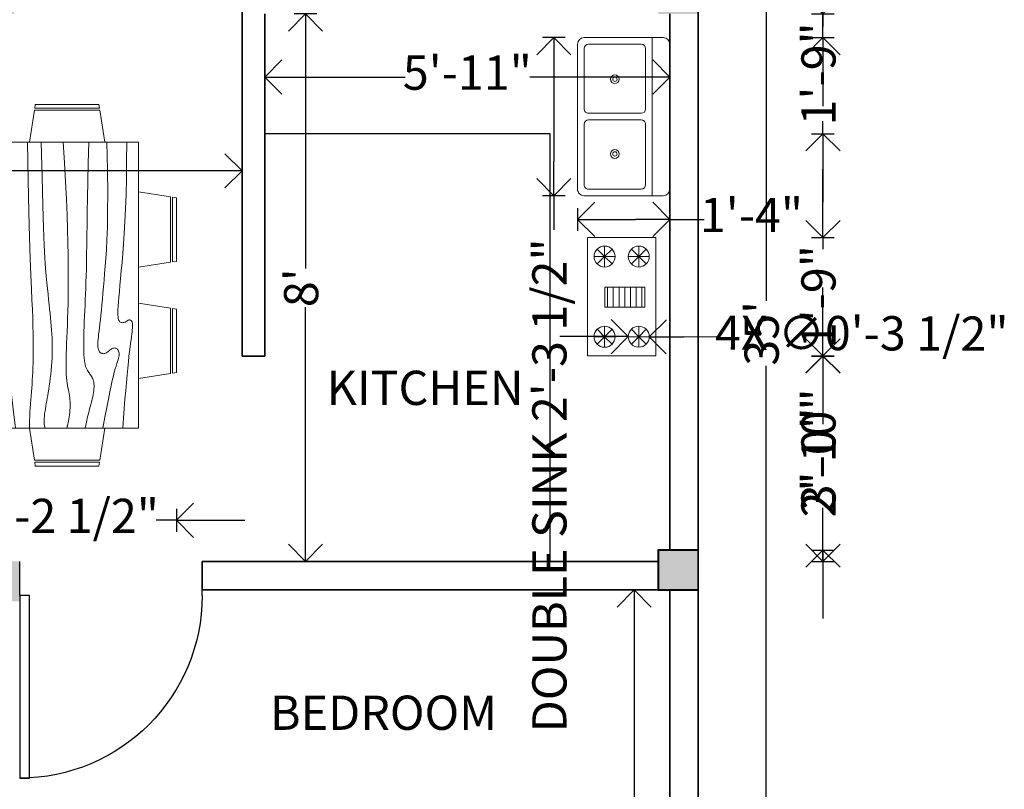
# Model space of a CAD drawing. Units: inches. Extents: x 261 to 714, y 97 to 573.
# Tile 4 of 5: x 541 to 714, y 253 to 388. Entities that reach past the tile are written whole.
import ezdxf

# ---------------------------------------------------------------- set-up
doc = ezdxf.new("R2010")
doc.units = ezdxf.units.IN
for name, color, linetype, lineweight in [('A-ANNO-DIMS', 2, 'Continuous', 18), ('A-AREA-IDEN', 7, 'Continuous', 25), ('A-COLS', 182, 'Continuous', 40), ('A-COLS-PATT', 172, 'Continuous', 13), ('A-DOOR', 182, 'Continuous', 25), ('A-EQPM', 8, 'Continuous', 18), ('A-FLOR-CASE', 182, 'Continuous', 25), ('A-FLOR-FIXT', 8, 'Continuous', 18), ('A-FURN', 8, 'Continuous', 18), ('A-WALL', 182, 'Continuous', 35)]:
    doc.layers.add(name, color=color, linetype=linetype, lineweight=lineweight)
doc.styles.get("Standard").update_dxf_attribs({"font": 'arial.ttf'})
doc.dimstyles.new('ISO-25', dxfattribs={"dimtxt": 6, "dimasz": 6, "dimexe": 2, "dimexo": 2, "dimtad": 0, "dimdec": 1, "dimlunit": 3, "dimtxsty": 'Standard', "dimblk": 'OPEN90', "dimcen": 2.5, "dimclrd": 1, "dimclre": 1, "dimclrt": 1, "dimadec": 0, "dimazin": 0, "dimtfac": 1, "dimtdec": 1, "dimtmove": 0, "dimatfit": 3, "dimfxl": 2, "dimfxlon": 1, "dimarcsym": 0})

# ---------------------------------------------------------------- blocks, each defined once
blk = doc.blocks.new('*U5')
for p, q in [((0, 0), (0, -6)), ((32, 0), (32, -6))]:
    blk.add_line(p, q)
blk.add_lwpolyline([(0, 0), (0, 32), (1.75, 32), (1.75, 0)], close=True)
blk.add_arc((0, 0), 32, 0, 90)
blk = doc.blocks.new('_Open90')
at = {"color": 0, "linetype": 'ByBlock', "lineweight": -2}
for p, q in [((-0.5, 0.5), (0, 0)), ((0, 0), (-1, 0)), ((0, 0), (-0.5, -0.5))]:
    blk.add_line(p, q, dxfattribs=at)
blk = doc.blocks.new('*D15')
at = {"layer": 'A-ANNO-DIMS', "color": 0, "lineweight": -2, "transparency": 16777216}
for p, q in [((352.9, 361.16), (352.9, 359.16)), ((358.9, 361.16), (453.42, 361.16)), ((573.9, 361.16), (479.38, 361.16)), ((579.9, 361.16), (579.9, 359.16))]:
    blk.add_line(p, q, dxfattribs=at)
at = {"layer": 'Defpoints', "color": 0, "transparency": 16777216}
for p in [(352.9, 361.54), (579.9, 361.54), (579.9, 361.16)]:
    blk.add_point(p, dxfattribs=at)
at = {"layer": 'A-ANNO-DIMS', "color": 0, "lineweight": -2, "transparency": 16777216, "xscale": 6, "yscale": 6, "zscale": 6, "rotation": 180}
blk.add_blockref('_Open90', (352.9, 361.16), dxfattribs=at)
at = {"layer": 'A-ANNO-DIMS', "color": 0, "lineweight": -2, "transparency": 16777216, "xscale": 6, "yscale": 6, "zscale": 6}
blk.add_blockref('_Open90', (579.9, 361.16), dxfattribs=at)
at = {"layer": 'A-ANNO-DIMS', "color": 0, "transparency": 16777216, "insert": (466.4, 361.16), "char_height": 6, "attachment_point": 5}
blk.add_mtext('18\'-10"', dxfattribs=at)
blk = doc.blocks.new('*D17')
at = {"layer": 'A-ANNO-DIMS', "color": 0, "lineweight": -2, "transparency": 16777216}
for p, q in [((593.03, 388.66), (589.03, 388.66)), ((591.03, 382.66), (591.03, 344.05)), ((591.03, 298.66), (591.03, 337.27)), ((593.03, 292.66), (589.03, 292.66))]:
    blk.add_line(p, q, dxfattribs=at)
at = {"layer": 'Defpoints', "color": 0, "transparency": 16777216}
for p in [(649.85, 388.66), (591.03, 292.66), (649.85, 292.66)]:
    blk.add_point(p, dxfattribs=at)
at = {"layer": 'A-ANNO-DIMS', "color": 0, "lineweight": -2, "transparency": 16777216, "xscale": 6, "yscale": 6, "zscale": 6}
for p, rotation in [((591.03, 388.66), 90), ((591.03, 292.66), 270)]:
    blk.add_blockref('_Open90', p, dxfattribs=dict(at, rotation=rotation))
at = {"layer": 'A-ANNO-DIMS', "color": 0, "transparency": 16777216, "insert": (591.03, 340.66), "char_height": 6, "attachment_point": 5, "rotation": 90}
blk.add_mtext("8'", dxfattribs=at)
blk = doc.blocks.new('*D18')
at = {"layer": 'A-ANNO-DIMS', "color": 0, "lineweight": -2, "transparency": 16777216}
for p, q in [((583.9, 375.6), (583.9, 379.6)), ((654.9, 375.6), (654.9, 379.6)), ((589.9, 377.6), (608.47, 377.6)), ((648.9, 377.6), (630.33, 377.6))]:
    blk.add_line(p, q, dxfattribs=at)
at = {"layer": 'Defpoints', "color": 0, "transparency": 16777216}
for p in [(654.9, 377.6), (583.9, 358.66), (654.9, 358.66)]:
    blk.add_point(p, dxfattribs=at)
at = {"layer": 'A-ANNO-DIMS', "color": 0, "lineweight": -2, "transparency": 16777216, "xscale": 6, "yscale": 6, "zscale": 6, "rotation": 180}
blk.add_blockref('_Open90', (583.9, 377.6), dxfattribs=at)
at = {"layer": 'A-ANNO-DIMS', "color": 0, "lineweight": -2, "transparency": 16777216, "xscale": 6, "yscale": 6, "zscale": 6}
blk.add_blockref('_Open90', (654.9, 377.6), dxfattribs=at)
at = {"layer": 'A-ANNO-DIMS', "color": 0, "transparency": 16777216, "insert": (619.4, 377.6), "char_height": 6, "attachment_point": 5}
blk.add_mtext('5\'-11"', dxfattribs=at)
blk = doc.blocks.new('*D21')
at = {"layer": 'A-ANNO-DIMS', "color": 0, "lineweight": -2, "transparency": 16777216}
for p, q in [((646.66, 287.66), (650.66, 287.66)), ((648.66, 281.66), (648.66, 233.09)), ((648.66, 173.66), (648.66, 222.22)), ((646.66, 167.66), (650.66, 167.66))]:
    blk.add_line(p, q, dxfattribs=at)
at = {"layer": 'Defpoints', "color": 0, "transparency": 16777216}
for p in [(643.84, 287.66), (643.84, 167.66), (648.66, 167.66)]:
    blk.add_point(p, dxfattribs=at)
at = {"layer": 'A-ANNO-DIMS', "color": 0, "lineweight": -2, "transparency": 16777216, "xscale": 6, "yscale": 6, "zscale": 6}
for p, rotation in [((648.66, 287.66), 90), ((648.66, 167.66), 270)]:
    blk.add_blockref('_Open90', p, dxfattribs=dict(at, rotation=rotation))
at = {"layer": 'A-ANNO-DIMS', "color": 0, "transparency": 16777216, "insert": (648.66, 227.66), "char_height": 6, "attachment_point": 5, "rotation": 90}
blk.add_mtext("10'", dxfattribs=at)
blk = doc.blocks.new('Sink-double - 36 in top')
for p, q in [((-18, -4), (18, -4)), ((-0.75, -18.5), (-0.75, -6.5)), ((0.75, -6.5), (0.75, -18.5))]:
    blk.add_line(p, q)
for points in [[(-16.5, 0), (16.5, 0)], [(-18, -19.5), (-18, -1.5)], [(18, -1.5), (18, -19.5)], [(-16.5, -18.5), (-16.5, -6.5)], [(-15.5, -5.5), (-1.75, -5.5)], [(1.75, -5.5), (15.5, -5.5)], [(16.5, -6.5), (16.5, -18.5)], [(-1.75, -19.5), (-15.5, -19.5)], [(15.5, -19.5), (1.75, -19.5)], [(16.5, -21), (-16.5, -21)]]:
    blk.add_lwpolyline(points)
for centre, radius in [((-8.5, -12.5), 1), ((-8.5, -12.5), 0.5), ((8.5, -12.5), 1), ((8.5, -12.5), 0.5)]:
    blk.add_circle(centre, radius)
for centre, radius, start, end in [((-16.5, -1.5), 1.5, 90, 180), ((16.5, -1.5), 1.5, 0, 90), ((-15.5, -6.5), 1, 90, 180), ((-1.75, -6.5), 1, 0, 90), ((1.75, -6.5), 1, 90, 180), ((15.5, -6.5), 1, 0, 90), ((-16.5, -19.5), 1.5, 180, 270), ((-15.5, -18.5), 1, 180, 270), ((-1.75, -18.5), 1, 270, 0), ((1.75, -18.5), 1, 180, 270), ((15.5, -18.5), 1, 270, 0), ((16.5, -19.5), 1.5, 270, 0)]:
    blk.add_arc(centre, radius, start, end)
blk = doc.blocks.new('Dining Set - 36 x 72 in.')
for p, q in [((-22, 27.5), (-22.1562, 26.50042)), ((-22, 27.5), (-6, 27.5)), ((-5.8437, 26.49966), (-6, 27.5)), ((6, 27.5), (5.8438, 26.50042)), ((6, 27.5), (22, 27.5)), ((22.1563, 26.49966), (22, 27.5)), ((-22.2343, 26.00059), (-23.4847, 17.99762)), ((-22.2304, 26), (-5.7608, 26)), ((-5.8416, 26.5), (-22.1534, 26.5)), ((-4.5152, 17.99762), (-5.7655, 25.99926)), ((5.7657, 26.00059), (4.5153, 17.99762)), ((5.7696, 26), (22.2392, 26)), ((22.1584, 26.5), (5.8466, 26.5)), ((23.4848, 17.99762), (22.2345, 25.99926)), ((36, 18), (-36, 18)), ((-36, 18), (-36, -18)), ((36, -18), (36, 18)), ((-45.5, 8), (-44.5004, 8.15617)), ((-45.5, 8), (-45.5, -8)), ((-44.5, -8.15843), (-44.5, 8.15338)), ((-44.0006, 8.23428), (-35.9976, 9.48474)), ((-44, 8.23041), (-44, -8.23915)), ((44.0006, 8.23428), (35.9976, 9.48474)), ((44, 8.23041), (44, -8.23915)), ((44.5, -8.15843), (44.5, 8.15338)), ((45.5, 8), (44.5005, 8.15617)), ((45.5, 8), (45.5, -8)), ((-44.4997, -8.15631), (-45.5, -8)), ((-35.9976, -9.48476), (-43.9993, -8.2345)), ((35.9976, -9.48476), (43.9993, -8.2345)), ((44.4997, -8.15631), (45.5, -8)), ((-36, -18), (36, -18)), ((-22.2343, -26.0006), (-23.4847, -17.99762)), ((-4.5152, -17.99762), (-5.7655, -25.99928)), ((5.7657, -26.0006), (4.5153, -17.99762)), ((23.4848, -17.99762), (22.2345, -25.99928)), ((-22.2304, -26), (-5.7608, -26)), ((-22, -27.5), (-22.1562, -26.50044)), ((-5.8416, -26.5), (-22.1534, -26.5)), ((-5.8437, -26.49967), (-6, -27.5)), ((5.7696, -26), (22.2392, -26)), ((6, -27.5), (5.8438, -26.50044)), ((22.1584, -26.5), (5.8466, -26.5)), ((22.1563, -26.49967), (22, -27.5)), ((-22, -27.5), (-6, -27.5)), ((6, -27.5), (22, -27.5))]:
    blk.add_line(p, q)
for points in [[(-36, 15), (-31.1772, 14.97754), (-26.8079, 14.91406), (-22.8538, 14.81543), (-19.276, 14.6875), (-16.0362, 14.53613), (-13.0957, 14.36718), (-10.4159, 14.18652), (-7.9583, 14), (-5.6904, 13.81315), (-3.6035, 13.63021), (-1.6954, 13.45508), (0.0365, 13.29166), (1.5945, 13.14388), (2.9811, 13.01562), (4.1988, 12.9108), (5.25, 12.83333), (6.1393, 12.78613), (6.8802, 12.76823), (7.4883, 12.77767), (7.9792, 12.8125), (8.3685, 12.87077), (8.6719, 12.95052), (8.9049, 13.0498), (9.0833, 13.16666), (9.2205, 13.29899), (9.3216, 13.44401), (9.3895, 13.59879), (9.4271, 13.76041), (9.4373, 13.92594), (9.4232, 14.09245), (9.3875, 14.257), (9.3333, 14.41666), (9.2638, 14.56917), (9.1836, 14.71484), (9.0975, 14.85465), (9.0104, 14.98958), (8.9272, 15.1206), (8.8529, 15.2487), (8.7922, 15.37483), (8.75, 15.5), (8.7305, 15.62467), (8.7344, 15.74739), (8.7617, 15.86621), (8.8125, 15.97916), (8.8867, 16.08431), (8.9844, 16.17968), (9.1055, 16.26334), (9.25, 16.33333), (9.4189, 16.38802), (9.6172, 16.42708), (9.8506, 16.45052), (10.125, 16.45833), (10.4463, 16.45052), (10.8203, 16.42708), (11.2529, 16.38802), (11.75, 16.33333), (12.3184, 16.26318), (12.9694, 16.17838), (13.7151, 16.07991), (14.5677, 15.96875), (15.5395, 15.84586), (16.6426, 15.71224), (17.8893, 15.56884), (19.2917, 15.41666), (20.859, 15.25667), (22.5879, 15.08984), (24.4721, 14.91715), (26.5052, 14.73958), (28.6809, 14.5581), (30.9929, 14.3737), (33.4347, 14.18733), (36, 14)], [(-36, 10), (-28.9766, 10.14274), (-23.1725, 10.20442), (-18.4241, 10.19775), (-14.5677, 10.13541), (-11.4399, 10.03011), (-8.877, 9.89453), (-6.7154, 9.74137), (-4.7917, 9.58333), (-2.9698, 9.43082), (-1.2246, 9.28515), (0.4415, 9.14534), (2.026, 9.01041), (3.5266, 8.87939), (4.9408, 8.7513), (6.266, 8.62516), (7.5, 8.5), (8.6411, 8.37549), (9.6914, 8.2539), (10.6538, 8.13818), (11.5312, 8.03125), (12.3267, 7.93603), (13.043, 7.85547), (13.6831, 7.79248), (14.25, 7.75), (14.7471, 7.7303), (15.1797, 7.73307), (15.5537, 7.75732), (15.875, 7.80208), (16.1494, 7.86637), (16.3828, 7.94922), (16.5811, 8.04964), (16.75, 8.16666), (16.8944, 8.29915), (17.0143, 8.44531), (17.1089, 8.60319), (17.1771, 8.77083), (17.218, 8.94629), (17.2305, 9.1276), (17.2137, 9.31282), (17.1667, 9.5), (17.0895, 9.6875), (16.987, 9.875), (16.8649, 10.0625), (16.7292, 10.25), (16.5856, 10.4375), (16.4401, 10.625), (16.2985, 10.8125), (16.1667, 11), (16.05, 11.18733), (15.9518, 11.3737), (15.8752, 11.5581), (15.8229, 11.73958), (15.798, 11.91715), (15.8034, 12.08984), (15.842, 12.25667), (15.9167, 12.41666), (16.0295, 12.56836), (16.1784, 12.70833), (16.3605, 12.83268), (16.5729, 12.9375), (16.8127, 13.01888), (17.0768, 13.07291), (17.3625, 13.0957), (17.6667, 13.08333), (17.9894, 13.03312), (18.3418, 12.94726), (18.7382, 12.82918), (19.1927, 12.68229), (19.7195, 12.51001), (20.3327, 12.31575), (21.0465, 12.10294), (21.875, 11.875), (22.8357, 11.63354), (23.959, 11.37304), (25.2786, 11.08618), (26.8282, 10.76562), (28.6414, 10.40405), (30.752, 9.99414), (33.1936, 9.52856), (36, 9)], [(-36, 5.5), (-30.7157, 5.3348), (-26.069, 5.20963), (-21.9946, 5.11767), (-18.4271, 5.05208), (-15.3009, 5.00602), (-12.5508, 4.97265), (-10.1112, 4.94515), (-7.9167, 4.91666), (-5.909, 4.88167), (-4.0586, 4.83984), (-2.3429, 4.79215), (-0.7396, 4.73958), (0.7739, 4.6831), (2.22, 4.6237), (3.6213, 4.56233), (5, 4.5), (6.373, 4.43782), (7.7344, 4.3776), (9.0723, 4.32129), (10.375, 4.27083), (11.6309, 4.22819), (12.8281, 4.19531), (13.9551, 4.17415), (15, 4.16666), (15.954, 4.17448), (16.819, 4.19791), (17.6001, 4.23698), (18.3021, 4.29166), (18.9299, 4.36198), (19.4883, 4.44791), (19.9823, 4.54948), (20.4167, 4.66666), (20.7969, 4.79899), (21.1302, 4.94401), (21.4245, 5.09879), (21.6875, 5.26041), (21.9271, 5.42594), (22.1511, 5.59245), (22.3672, 5.757), (22.5834, 5.91666), (22.8065, 6.06868), (23.0404, 6.21093), (23.2879, 6.34147), (23.5521, 6.45833), (23.8358, 6.55957), (24.142, 6.64323), (24.4735, 6.70735), (24.8334, 6.75), (25.2235, 6.76969), (25.642, 6.76692), (26.0858, 6.74267), (26.5521, 6.69791), (27.0379, 6.63362), (27.5404, 6.55078), (28.0565, 6.45036), (28.5834, 6.33333), (29.1242, 6.19987), (29.7071, 6.04687), (30.3661, 5.87044), (31.1354, 5.66666), (32.0493, 5.43164), (33.142, 5.16146), (34.4475, 4.85221), (36, 4.5)], [(-36, -1), (-30.7915, -0.6591), (-26.0195, -0.38216), (-21.6519, -0.16284), (-17.6563, 0.00521), (-14.0005, 0.12833), (-10.6523, 0.21289), (-7.5796, 0.26522), (-4.75, 0.29166), (-2.134, 0.29793), (0.2878, 0.28711), (2.5317, 0.26163), (4.6146, 0.22396), (6.5529, 0.17651), (8.3633, 0.12174), (10.0623, 0.06209), (11.6667, 0), (13.1899, -0.06201), (14.6341, -0.1211), (15.9982, -0.17432), (17.2813, -0.21875), (18.4823, -0.25147), (19.6003, -0.26953), (20.6343, -0.27002), (21.5834, -0.25), (22.4481, -0.20768), (23.2357, -0.14584), (23.9549, -0.06836), (24.6146, 0.02083), (25.2235, 0.11784), (25.7904, 0.21875), (26.3241, 0.31966), (26.8334, 0.41666), (27.3265, 0.50618), (27.8099, 0.58593), (28.2894, 0.65397), (28.7709, 0.70833), (29.2601, 0.74707), (29.763, 0.76823), (30.2855, 0.76985), (30.8334, 0.75), (31.4088, 0.70784), (31.9994, 0.64713), (32.589, 0.57275), (33.1615, 0.48958), (33.7008, 0.4025), (34.1908, 0.3164), (34.6153, 0.23616), (34.9584, 0.16666), (35.2099, 0.11165), (35.3848, 0.07031), (35.504, 0.04069), (35.5886, 0.02083), (35.6594, 0.00879), (35.7377, 0.0026), (35.8442, 0.00032), (36, 0)], [(-36, -6.5), (-27.1843, -6.31267), (-20.084, -6.1263), (-14.469, -5.9419), (-10.1094, -5.76042), (-6.7752, -5.58285), (-4.2363, -5.41016), (-2.2629, -5.24333), (-0.625, -5.08334), (0.8708, -4.93099), (2.2715, -4.78646), (3.5872, -4.64974), (4.8281, -4.52084), (6.0046, -4.39974), (7.127, -4.28646), (8.2053, -4.18099), (9.25, -4.08334), (10.2705, -3.99382), (11.2734, -3.91407), (12.2647, -3.84603), (13.25, -3.79167), (14.2354, -3.75293), (15.2266, -3.73177), (16.2295, -3.73015), (17.25, -3.75), (18.2912, -3.79248), (19.3451, -3.85547), (20.4009, -3.93604), (21.4479, -4.03125), (22.4754, -4.13819), (23.4727, -4.25391), (24.4289, -4.37549), (25.3334, -4.5), (26.1785, -4.62492), (26.9694, -4.74935), (27.7145, -4.87281), (28.4219, -4.99479), (29.1, -5.11483), (29.7572, -5.23242), (30.4016, -5.34709), (31.0417, -5.45834), (31.6837, -5.56437), (32.3262, -5.65821), (32.9658, -5.73153), (33.599, -5.77604), (34.2224, -5.78345), (34.8327, -5.74545), (35.4264, -5.65373), (36, -5.5)], [(-36, -10), (-26.4022, -9.81299), (-18.4675, -9.62891), (-11.9839, -9.45069), (-6.7396, -9.28125), (-2.5226, -9.12354), (0.8789, -8.98047), (3.6769, -8.85498), (6.0833, -8.75), (8.2767, -8.66765), (10.3021, -8.60677), (12.1712, -8.56543), (13.8958, -8.54167), (15.4876, -8.53353), (16.9583, -8.53907), (18.3197, -8.55632), (19.5834, -8.58334), (20.7616, -8.61841), (21.8685, -8.66081), (22.9188, -8.71004), (23.9271, -8.76563), (24.9081, -8.82707), (25.8763, -8.89388), (26.8465, -8.96558), (27.8334, -9.04167), (28.8474, -9.12118), (29.8828, -9.20117), (30.93, -9.27824), (31.9792, -9.34896), (33.0205, -9.40991), (34.0443, -9.45768), (35.0407, -9.48885), (36, -9.5)], [(-36, -14.5), (-30.0881, -14.33513), (-25.0332, -14.21224), (-20.7312, -14.12647), (-17.0781, -14.07292), (-13.97, -14.04671), (-11.3027, -14.04297), (-8.9724, -14.05681), (-6.875, -14.08334), (-4.9224, -14.11833), (-3.0905, -14.16016), (-1.3709, -14.20785), (0.2448, -14.26042), (1.7647, -14.3169), (3.1973, -14.3763), (4.5507, -14.43767), (5.8333, -14.5), (7.0554, -14.5621), (8.235, -14.62175), (9.3922, -14.67652), (10.5469, -14.72396), (11.7192, -14.76164), (12.929, -14.78711), (14.1965, -14.79794), (15.5417, -14.79167), (16.9933, -14.76424), (18.6152, -14.70508), (20.4804, -14.60197), (22.6615, -14.44271), (25.2312, -14.21509), (28.2624, -13.9069), (31.8277, -13.50594), (36, -13)]]:
    blk.add_lwpolyline(points)
blk = doc.blocks.new('*D35')
at = {"layer": 'A-ANNO-DIMS', "color": 0, "lineweight": -2, "transparency": 16777216}
for p, q in [((669.78, 542.66), (673.78, 542.66)), ((671.78, 536.66), (671.78, 338.37)), ((671.78, 128.66), (671.78, 326.94)), ((669.78, 122.66), (673.78, 122.66))]:
    blk.add_line(p, q, dxfattribs=at)
at = {"layer": 'Defpoints', "color": 0, "transparency": 16777216}
for p in [(659.9, 542.66), (659.9, 122.66), (671.78, 122.66)]:
    blk.add_point(p, dxfattribs=at)
at = {"layer": 'A-ANNO-DIMS', "color": 0, "lineweight": -2, "transparency": 16777216, "xscale": 6, "yscale": 6, "zscale": 6}
for p, rotation in [((671.78, 542.66), 90), ((671.78, 122.66), 270)]:
    blk.add_blockref('_Open90', p, dxfattribs=dict(at, rotation=rotation))
at = {"layer": 'A-ANNO-DIMS', "color": 0, "transparency": 16777216, "insert": (671.78, 332.66), "char_height": 6, "attachment_point": 5, "rotation": 90}
blk.add_mtext("35'", dxfattribs=at)
blk = doc.blocks.new('COOKTOP-BURNER')
for p, q in [((1.84, 0), (1.84, 3.67)), ((0, 1.84), (3.67, 1.84)), ((0.54, 3.14), (1.84, 1.84)), ((0.54, 0.54), (1.84, 1.84)), ((3.13, 3.14), (1.84, 1.84)), ((3.13, 0.54), (1.84, 1.84))]:
    blk.add_line(p, q)
blk.add_circle((1.84, 1.84), 1.84)
blk = doc.blocks.new('COLUMN-7IN-SIDE-EDGE')
blk.add_lwpolyline([(7, 7), (0, 7), (0, 2), (0, 0), (2, 0), (7, 0)])
blk = doc.blocks.new('*D49')
at = {"layer": 'A-ANNO-DIMS', "color": 1, "lineweight": -2, "transparency": 16777216}
for p, q in [((636.57, 384.52), (632.57, 384.52)), ((634.57, 378.52), (634.57, 362.79)), ((636.57, 356.79), (632.57, 356.79)), ((634.57, 356.79), (634.57, 350.79))]:
    blk.add_line(p, q, dxfattribs=at)
at = {"layer": 'Defpoints', "color": 0, "transparency": 16777216}
for p in [(638.73, 384.52), (634.57, 356.79), (638.73, 356.79)]:
    blk.add_point(p, dxfattribs=at)
at = {"layer": 'A-ANNO-DIMS', "color": 1, "lineweight": -2, "transparency": 16777216, "xscale": 6, "yscale": 6, "zscale": 6}
for p, rotation in [((634.57, 384.52), 90), ((634.57, 356.79), 270)]:
    blk.add_blockref('_Open90', p, dxfattribs=dict(at, rotation=rotation))
at = {"layer": 'A-ANNO-DIMS', "color": 1, "transparency": 16777216, "insert": (634.57, 306), "char_height": 6, "attachment_point": 5, "rotation": 90}
blk.add_mtext('DOUBLE SINK 2\'-3 1/2"', dxfattribs=at)
blk = doc.blocks.new('*D50')
at = {"layer": 'A-ANNO-DIMS', "color": 1, "lineweight": -2, "transparency": 16777216}
for p, q in [((638.73, 354.63), (638.73, 350.63)), ((654.9, 354.63), (654.9, 350.63)), ((644.73, 352.63), (648.9, 352.63)), ((654.9, 352.63), (660.9, 352.63))]:
    blk.add_line(p, q, dxfattribs=at)
at = {"layer": 'Defpoints', "color": 0, "transparency": 16777216}
for p in [(638.73, 356.79), (654.9, 356.79), (654.9, 352.63)]:
    blk.add_point(p, dxfattribs=at)
at = {"layer": 'A-ANNO-DIMS', "color": 1, "lineweight": -2, "transparency": 16777216, "xscale": 6, "yscale": 6, "zscale": 6, "rotation": 180}
blk.add_blockref('_Open90', (638.73, 352.63), dxfattribs=at)
at = {"layer": 'A-ANNO-DIMS', "color": 1, "lineweight": -2, "transparency": 16777216, "xscale": 6, "yscale": 6, "zscale": 6}
blk.add_blockref('_Open90', (654.9, 352.63), dxfattribs=at)
at = {"layer": 'A-ANNO-DIMS', "color": 1, "transparency": 16777216, "insert": (669.22, 352.63), "char_height": 6, "attachment_point": 5}
blk.add_mtext('1\'-4"', dxfattribs=at)
blk = doc.blocks.new('*D52')
at = {"layer": 'A-ANNO-DIMS', "color": 1, "lineweight": -2, "transparency": 16777216}
for p, q in [((530.06, 301.87), (530.06, 297.87)), ((568.39, 301.87), (568.39, 297.87)), ((524.06, 299.87), (518.06, 299.87)), ((530.06, 299.87), (533.63, 299.87)), ((568.39, 299.87), (564.81, 299.87)), ((574.39, 299.87), (580.39, 299.87))]:
    blk.add_line(p, q, dxfattribs=at)
at = {"layer": 'Defpoints', "color": 0, "transparency": 16777216}
for p in [(530.06, 309.39), (568.39, 309.39), (568.39, 299.87)]:
    blk.add_point(p, dxfattribs=at)
at = {"layer": 'A-ANNO-DIMS', "color": 1, "lineweight": -2, "transparency": 16777216, "xscale": 6, "yscale": 6, "zscale": 6}
blk.add_blockref('_Open90', (530.06, 299.87), dxfattribs=at)
at = {"layer": 'A-ANNO-DIMS', "color": 1, "lineweight": -2, "transparency": 16777216, "xscale": 6, "yscale": 6, "zscale": 6, "rotation": 180}
blk.add_blockref('_Open90', (568.39, 299.87), dxfattribs=at)
at = {"layer": 'A-ANNO-DIMS', "color": 1, "transparency": 16777216, "insert": (549.22, 299.87), "char_height": 6, "attachment_point": 5}
blk.add_mtext('3\'-2 1/2"', dxfattribs=at)
blk = doc.blocks.new('*D63')
at = {"layer": 'A-ANNO-DIMS', "color": 1, "lineweight": -2, "transparency": 16777216}
for p, q in [((540.9, 102.81), (540.9, 98.81)), ((572.9, 102.81), (572.9, 98.81)), ((546.9, 100.81), (548.25, 100.81)), ((566.9, 100.81), (565.55, 100.81))]:
    blk.add_line(p, q, dxfattribs=at)
at = {"layer": 'Defpoints', "color": 0, "transparency": 16777216}
for p in [(540.9, 287.66), (572.9, 287.66), (572.9, 100.81)]:
    blk.add_point(p, dxfattribs=at)
at = {"layer": 'A-ANNO-DIMS', "color": 1, "lineweight": -2, "transparency": 16777216, "xscale": 6, "yscale": 6, "zscale": 6, "rotation": 180}
blk.add_blockref('_Open90', (540.9, 100.81), dxfattribs=at)
at = {"layer": 'A-ANNO-DIMS', "color": 1, "lineweight": -2, "transparency": 16777216, "xscale": 6, "yscale": 6, "zscale": 6}
blk.add_blockref('_Open90', (572.9, 100.81), dxfattribs=at)
at = {"layer": 'A-ANNO-DIMS', "color": 1, "transparency": 16777216, "insert": (556.9, 100.81), "char_height": 6, "attachment_point": 5}
blk.add_mtext('2\'-8"', dxfattribs=at)
blk = doc.blocks.new('*D64')
at = {"layer": 'A-ANNO-DIMS', "color": 1, "lineweight": -2, "transparency": 16777216}
for p, q in [((572.9, 102.81), (572.9, 98.81)), ((652.88, 102.81), (652.88, 98.81)), ((578.9, 100.81), (604.28, 100.81)), ((646.88, 100.81), (621.51, 100.81))]:
    blk.add_line(p, q, dxfattribs=at)
at = {"layer": 'Defpoints', "color": 0, "transparency": 16777216}
for p in [(572.9, 287.66), (652.88, 287.66), (652.88, 100.81)]:
    blk.add_point(p, dxfattribs=at)
at = {"layer": 'A-ANNO-DIMS', "color": 1, "lineweight": -2, "transparency": 16777216, "xscale": 6, "yscale": 6, "zscale": 6, "rotation": 180}
blk.add_blockref('_Open90', (572.9, 100.81), dxfattribs=at)
at = {"layer": 'A-ANNO-DIMS', "color": 1, "lineweight": -2, "transparency": 16777216, "xscale": 6, "yscale": 6, "zscale": 6}
blk.add_blockref('_Open90', (652.88, 100.81), dxfattribs=at)
at = {"layer": 'A-ANNO-DIMS', "color": 1, "transparency": 16777216, "insert": (612.89, 100.81), "char_height": 6, "attachment_point": 5}
blk.add_mtext('6\'-8"', dxfattribs=at)
blk = doc.blocks.new('*D68')
at = {"layer": 'A-ANNO-DIMS', "color": 1, "lineweight": -2, "transparency": 16777216}
for p, q in [((633.9, 562.51), (633.9, 566.51)), ((654.9, 562.51), (654.9, 566.51)), ((627.9, 564.51), (621.9, 564.51)), ((633.9, 564.51), (636.09, 564.51)), ((654.9, 564.51), (652.72, 564.51)), ((660.9, 564.51), (666.9, 564.51))]:
    blk.add_line(p, q, dxfattribs=at)
at = {"layer": 'Defpoints', "color": 0, "transparency": 16777216}
for p in [(654.9, 564.51), (654.9, 294.66), (633.9, 292.66)]:
    blk.add_point(p, dxfattribs=at)
at = {"layer": 'A-ANNO-DIMS', "color": 1, "lineweight": -2, "transparency": 16777216, "xscale": 6, "yscale": 6, "zscale": 6}
blk.add_blockref('_Open90', (633.9, 564.51), dxfattribs=at)
at = {"layer": 'A-ANNO-DIMS', "color": 1, "lineweight": -2, "transparency": 16777216, "xscale": 6, "yscale": 6, "zscale": 6, "rotation": 180}
blk.add_blockref('_Open90', (654.9, 564.51), dxfattribs=at)
at = {"layer": 'A-ANNO-DIMS', "color": 1, "transparency": 16777216, "insert": (644.4, 564.51), "char_height": 6, "attachment_point": 5}
blk.add_mtext('1\'-9"', dxfattribs=at)
blk = doc.blocks.new('*D69')
at = {"layer": 'A-ANNO-DIMS', "color": 1, "lineweight": -2, "transparency": 16777216}
for p, q in [((579.9, 102.81), (579.9, 98.81)), ((583.9, 102.81), (583.9, 98.81)), ((573.9, 100.81), (567.9, 100.81)), ((579.9, 100.81), (583.9, 100.81)), ((589.9, 100.81), (595.9, 100.81))]:
    blk.add_line(p, q, dxfattribs=at)
at = {"layer": 'Defpoints', "color": 0, "transparency": 16777216}
for p in [(579.9, 328.66), (583.9, 328.66), (583.9, 100.81)]:
    blk.add_point(p, dxfattribs=at)
at = {"layer": 'A-ANNO-DIMS', "color": 1, "lineweight": -2, "transparency": 16777216, "xscale": 6, "yscale": 6, "zscale": 6}
blk.add_blockref('_Open90', (579.9, 100.81), dxfattribs=at)
at = {"layer": 'A-ANNO-DIMS', "color": 1, "lineweight": -2, "transparency": 16777216, "xscale": 6, "yscale": 6, "zscale": 6, "rotation": 180}
blk.add_blockref('_Open90', (583.9, 100.81), dxfattribs=at)
at = {"layer": 'A-ANNO-DIMS', "color": 1, "transparency": 16777216, "insert": (604.5, 100.81), "char_height": 6, "attachment_point": 5}
blk.add_mtext('0\'-4"', dxfattribs=at)
blk = doc.blocks.new('*D70')
at = {"layer": 'A-ANNO-DIMS', "color": 1, "lineweight": -2, "transparency": 16777216}
for p, q in [((679.75, 328.66), (683.75, 328.66)), ((681.75, 322.66), (681.75, 319.25)), ((681.75, 298.66), (681.75, 302.06)), ((679.75, 292.66), (683.75, 292.66))]:
    blk.add_line(p, q, dxfattribs=at)
at = {"layer": 'Defpoints', "color": 0, "transparency": 16777216}
for p in [(583.9, 328.66), (572.9, 292.66), (681.75, 292.66)]:
    blk.add_point(p, dxfattribs=at)
at = {"layer": 'A-ANNO-DIMS', "color": 1, "lineweight": -2, "transparency": 16777216, "xscale": 6, "yscale": 6, "zscale": 6}
for p, rotation in [((681.75, 328.66), 90), ((681.75, 292.66), 270)]:
    blk.add_blockref('_Open90', p, dxfattribs=dict(at, rotation=rotation))
at = {"layer": 'A-ANNO-DIMS', "color": 1, "transparency": 16777216, "insert": (681.75, 310.66), "char_height": 6, "attachment_point": 5, "rotation": 90}
blk.add_mtext('3\'-0"', dxfattribs=at)
blk = doc.blocks.new('*D72')
at = {"layer": 'A-ANNO-DIMS', "color": 1, "lineweight": -2, "transparency": 16777216}
for p, q in [((681.75, 394.66), (681.75, 400.66)), ((679.75, 388.66), (683.75, 388.66)), ((681.75, 388.66), (681.75, 386.47)), ((681.75, 367.66), (681.75, 369.84)), ((679.75, 367.66), (683.75, 367.66)), ((681.75, 361.66), (681.75, 355.66))]:
    blk.add_line(p, q, dxfattribs=at)
at = {"layer": 'Defpoints', "color": 0, "transparency": 16777216}
for p in [(583.9, 388.66), (681.75, 388.66), (583.9, 367.66)]:
    blk.add_point(p, dxfattribs=at)
at = {"layer": 'A-ANNO-DIMS', "color": 1, "lineweight": -2, "transparency": 16777216, "xscale": 6, "yscale": 6, "zscale": 6}
for p, rotation in [((681.75, 388.66), 270), ((681.75, 367.66), 90)]:
    blk.add_blockref('_Open90', p, dxfattribs=dict(at, rotation=rotation))
at = {"layer": 'A-ANNO-DIMS', "color": 1, "transparency": 16777216, "insert": (681.75, 378.16), "char_height": 6, "attachment_point": 5, "rotation": 90}
blk.add_mtext('1\'-9"', dxfattribs=at)
blk = doc.blocks.new('*D75')
at = {"layer": 'A-ANNO-DIMS', "color": 1, "lineweight": -2, "transparency": 16777216}
for p, q in [((640.47, 102.81), (640.47, 98.81)), ((652.46, 102.81), (652.46, 98.81)), ((634.47, 100.81), (628.47, 100.81)), ((640.47, 100.81), (652.46, 100.81)), ((658.46, 100.81), (664.46, 100.81))]:
    blk.add_line(p, q, dxfattribs=at)
at = {"layer": 'Defpoints', "color": 0, "transparency": 16777216}
for p in [(640.47, 328.71), (652.46, 328.71), (652.46, 100.81)]:
    blk.add_point(p, dxfattribs=at)
at = {"layer": 'A-ANNO-DIMS', "color": 1, "lineweight": -2, "transparency": 16777216, "xscale": 6, "yscale": 6, "zscale": 6}
blk.add_blockref('_Open90', (640.47, 100.81), dxfattribs=at)
at = {"layer": 'A-ANNO-DIMS', "color": 1, "lineweight": -2, "transparency": 16777216, "xscale": 6, "yscale": 6, "zscale": 6, "rotation": 180}
blk.add_blockref('_Open90', (652.46, 100.81), dxfattribs=at)
at = {"layer": 'A-ANNO-DIMS', "color": 1, "transparency": 16777216, "insert": (672.77, 100.81), "char_height": 6, "attachment_point": 5}
blk.add_mtext('1\'-0"', dxfattribs=at)
blk = doc.blocks.new('*D76')
at = {"layer": 'A-ANNO-DIMS', "color": 1, "lineweight": -2, "transparency": 16777216}
for p, q in [((681.75, 355.47), (681.75, 361.47)), ((679.75, 349.47), (683.75, 349.47)), ((681.75, 349.47), (681.75, 347.41)), ((681.75, 328.71), (681.75, 330.78)), ((679.75, 328.71), (683.75, 328.71)), ((681.75, 322.71), (681.75, 316.71))]:
    blk.add_line(p, q, dxfattribs=at)
at = {"layer": 'Defpoints', "color": 0, "transparency": 16777216}
for p in [(652.46, 349.47), (681.75, 349.47), (652.46, 328.71)]:
    blk.add_point(p, dxfattribs=at)
at = {"layer": 'A-ANNO-DIMS', "color": 1, "lineweight": -2, "transparency": 16777216, "xscale": 6, "yscale": 6, "zscale": 6}
for p, rotation in [((681.75, 349.47), 270), ((681.75, 328.71), 90)]:
    blk.add_blockref('_Open90', p, dxfattribs=dict(at, rotation=rotation))
at = {"layer": 'A-ANNO-DIMS', "color": 1, "transparency": 16777216, "insert": (681.75, 339.09), "char_height": 6, "attachment_point": 5, "rotation": 90}
blk.add_mtext('1\'-9"', dxfattribs=at)
blk = doc.blocks.new('*D77')
at = {"layer": 'A-ANNO-DIMS', "color": 1, "lineweight": -2, "transparency": 16777216}
for p, q in [((681.75, 334.71), (681.75, 340.71)), ((679.75, 328.71), (683.75, 328.71)), ((681.75, 328.71), (681.75, 322.67)), ((681.75, 294.66), (681.75, 300.7)), ((679.75, 294.66), (683.75, 294.66)), ((681.75, 288.66), (681.75, 282.66))]:
    blk.add_line(p, q, dxfattribs=at)
at = {"layer": 'Defpoints', "color": 0, "transparency": 16777216}
for p in [(652.46, 328.71), (652.88, 294.66), (681.75, 294.66)]:
    blk.add_point(p, dxfattribs=at)
at = {"layer": 'A-ANNO-DIMS', "color": 1, "lineweight": -2, "transparency": 16777216, "xscale": 6, "yscale": 6, "zscale": 6}
for p, rotation in [((681.75, 328.71), 270), ((681.75, 294.66), 90)]:
    blk.add_blockref('_Open90', p, dxfattribs=dict(at, rotation=rotation))
at = {"layer": 'A-ANNO-DIMS', "color": 1, "transparency": 16777216, "insert": (681.75, 311.69), "char_height": 6, "attachment_point": 5, "rotation": 90}
blk.add_mtext('2\'-10"', dxfattribs=at)
blk = doc.blocks.new('*D78')
at = {"layer": 'A-ANNO-DIMS', "color": 1, "lineweight": -2, "transparency": 16777216}
for p, q in [((681.75, 394.66), (681.75, 400.66)), ((679.75, 388.66), (683.75, 388.66)), ((681.75, 384.52), (681.75, 388.66)), ((679.75, 384.52), (683.75, 384.52)), ((681.75, 378.52), (681.75, 372.52))]:
    blk.add_line(p, q, dxfattribs=at)
at = {"layer": 'Defpoints', "color": 0, "transparency": 16777216}
for p in [(652.88, 388.66), (681.75, 388.66), (651.82, 384.52)]:
    blk.add_point(p, dxfattribs=at)
at = {"layer": 'A-ANNO-DIMS', "color": 1, "lineweight": -2, "transparency": 16777216, "xscale": 6, "yscale": 6, "zscale": 6}
for p, rotation in [((681.75, 388.66), 270), ((681.75, 384.52), 90)]:
    blk.add_blockref('_Open90', p, dxfattribs=dict(at, rotation=rotation))
at = {"layer": 'A-ANNO-DIMS', "color": 1, "transparency": 16777216, "insert": (681.75, 409.26), "char_height": 6, "attachment_point": 5, "rotation": 90}
blk.add_mtext('0\'-4"', dxfattribs=at)
blk = doc.blocks.new('*D83')
at = {"layer": 'A-ANNO-DIMS', "color": 1, "lineweight": -2, "transparency": 16777216}
for p, q in [((641.62, 332.1), (635.62, 332.12)), ((647.62, 332.08), (651.3, 332.06)), ((663.3, 332.01), (657.3, 332.04))]:
    blk.add_line(p, q, dxfattribs=at)
at = {"layer": 'Defpoints', "color": 0, "transparency": 16777216}
for p in [(647.62, 332.08), (651.3, 332.06)]:
    blk.add_point(p, dxfattribs=at)
at = {"layer": 'A-ANNO-DIMS', "color": 1, "lineweight": -2, "transparency": 16777216, "xscale": 6, "yscale": 6, "zscale": 6}
for p, rotation in [((647.62, 332.08), 359.764530157097), ((651.3, 332.06), 179.764530157097)]:
    blk.add_blockref('_Open90', p, dxfattribs=dict(at, rotation=rotation))
at = {"layer": 'A-ANNO-DIMS', "color": 1, "transparency": 16777216, "insert": (688.56, 331.91), "char_height": 6, "attachment_point": 5, "rotation": 359.7645}
blk.add_mtext('4X ∅0\'-3 1/2"', dxfattribs=at)

msp = doc.modelspace()

# ---------------------------------------------------------------- hatches: boundary and pattern name
at = {"layer": 'A-COLS-PATT'}
h = msp.add_hatch(color=256, dxfattribs=at)
h.dxf.hatch_style = 1
h.paths.add_polyline_path([(354.9, 542.66), (347.9, 542.66), (347.9, 535.66), (354.9, 535.66)])
h.paths.add_polyline_path([(539.9, 542.66), (532.9, 542.66), (532.9, 537.66), (532.9, 535.66), (534.9, 535.66), (539.9, 535.66), (539.9, 537.66)])
h.paths.add_polyline_path([(474.9, 542.66), (467.9, 542.66), (467.9, 537.66), (467.9, 535.66), (469.9, 535.66), (474.9, 535.66), (474.9, 537.66)])
h.paths.add_polyline_path([(659.9, 542.66), (652.9, 542.66), (652.9, 537.66), (652.9, 535.66), (654.9, 535.66), (659.9, 535.66)])
h.paths.add_polyline_path([(659.9, 395.66), (652.88, 395.66), (652.88, 390.66), (652.88, 388.66), (654.88, 388.66), (659.9, 388.66)])
h.paths.add_polyline_path([(539.9, 395.66), (532.9, 395.66), (532.9, 390.66), (532.9, 388.66), (534.9, 388.66), (539.9, 388.66), (539.9, 390.66)])
h.paths.add_polyline_path([(473.9, 395.66), (466.9, 395.66), (466.9, 394.66), (466.9, 388.66), (473.9, 388.66)])
h.paths.add_polyline_path([(354.9, 394.66), (347.9, 394.66), (347.9, 389.66), (347.9, 387.66), (349.9, 387.66), (354.9, 387.66), (354.9, 389.66)])
h.paths.add_polyline_path([(540.9, 292.66), (533.9, 292.66), (533.9, 287.66), (533.9, 285.66), (535.9, 285.66), (540.9, 285.66), (540.9, 287.66)])
h.paths.add_polyline_path([(659.9, 294.66), (652.88, 294.66), (652.88, 289.66), (652.88, 287.66), (654.88, 287.66), (659.9, 287.66)])
h.paths.add_polyline_path([(473.9, 292.66), (466.9, 292.66), (466.9, 287.66), (466.9, 285.66), (468.9, 285.66), (473.9, 285.66), (473.9, 287.66)])
h.paths.add_polyline_path([(354.9, 293.66), (347.9, 293.66), (347.9, 288.66), (347.9, 286.66), (349.9, 286.66), (354.9, 286.66), (354.9, 288.66)])
h.paths.add_polyline_path([(354.9, 129.66), (347.9, 129.66), (347.9, 124.66), (347.9, 122.66), (349.9, 122.66), (354.9, 122.66), (354.9, 124.66)])
h.paths.add_polyline_path([(354.9, 168.66), (347.9, 168.66), (347.9, 163.66), (347.9, 161.66), (349.9, 161.66), (354.9, 161.66), (354.9, 163.66)])
h.paths.add_polyline_path([(473.9, 169.69), (466.95, 169.69), (466.95, 164.69), (466.95, 162.69), (468.95, 162.69), (473.9, 162.69)])
h.paths.add_polyline_path([(475.9, 129.66), (468.9, 129.66), (468.9, 124.66), (468.9, 122.66), (470.9, 122.66), (475.9, 122.66), (475.9, 124.66)])
h.paths.add_polyline_path([(540.9, 129.66), (533.9, 129.66), (533.9, 124.66), (533.9, 122.66), (535.9, 122.66), (540.9, 122.66), (540.9, 124.66)])
h.paths.add_polyline_path([(540.9, 169.66), (533.9, 169.66), (533.9, 164.66), (533.9, 162.66), (535.9, 162.66), (540.9, 162.66), (540.9, 164.66)])
h.paths.add_polyline_path([(659.9, 169.66), (652.9, 169.66), (652.9, 164.66), (652.9, 162.66), (654.9, 162.66), (659.9, 162.66)])
h.paths.add_polyline_path([(659.9, 129.66), (652.9, 129.66), (652.9, 124.66), (652.9, 122.66), (654.9, 122.66), (659.9, 122.66)])

# ---------------------------------------------------------------- linework, layer by layer
at = {"layer": 'A-EQPM'}
for p, q in [((644, 340.73), (644, 337.25)), ((645, 340.73), (645, 337.25)), ((646, 340.73), (646, 337.25)), ((647, 340.73), (647, 337.25)), ((648, 340.73), (648, 337.25)), ((649.01, 340.73), (649.01, 337.25)), ((650.01, 340.73), (650.01, 337.25))]:
    msp.add_line(p, q, dxfattribs=at)
for points in [[(652.46, 349.47), (640.47, 349.47), (640.47, 328.71), (652.46, 328.71)], [(643.5, 340.73), (650.51, 340.73), (650.51, 337.25), (643.5, 337.25)]]:
    msp.add_lwpolyline(points, close=True, dxfattribs=at)
at = {"layer": 'A-FLOR-CASE'}
for p, q in [((633.9, 367.66), (583.9, 367.66)), ((633.9, 292.66), (633.9, 367.66))]:
    msp.add_line(p, q, dxfattribs=at)
at = {"layer": 'A-WALL'}
for p, q in [((659.9, 122.66), (659.9, 542.66)), ((579.9, 393.66), (579.9, 328.66)), ((583.9, 388.66), (583.9, 328.66)), ((654.9, 294.66), (654.9, 388.66)), ((583.9, 328.66), (579.9, 328.66)), ((572.9, 292.66), (572.9, 287.66)), ((572.9, 292.66), (652.88, 292.66)), ((572.9, 287.66), (654.9, 287.66)), ((654.9, 169.66), (654.9, 287.66))]:
    msp.add_line(p, q, dxfattribs=at)

# ---------------------------------------------------------------- block references
at = {"layer": 'A-COLS'}
msp.add_blockref('COLUMN-7IN-SIDE-EDGE', (652.88, 287.66), dxfattribs=at)
at = {"layer": 'A-DOOR', "xscale": -1, "rotation": 180}
msp.add_blockref('*U5', (540.9, 286.66), dxfattribs=at)
at = {"layer": 'A-EQPM'}
for p, rotation in [((641.63, 347.96), 269.9999999999964), ((647.62, 347.96), 270), ((641.63, 333.9), 269.9999999999964)]:
    msp.add_blockref('COOKTOP-BURNER', p, dxfattribs=dict(at, rotation=rotation))
msp.add_blockref('COOKTOP-BURNER', (647.62, 330.23), dxfattribs=at)
at = {"layer": 'A-FLOR-FIXT', "xscale": 0.7703624924072745, "yscale": 0.7703624924072745, "zscale": 0.7703624924072745, "rotation": 270}
msp.add_blockref('Sink-double - 36 in top', (654.9, 370.66), dxfattribs=at)
at = {"layer": 'A-FURN', "xscale": 0.6969524783132904, "yscale": 0.6969524783132904, "zscale": 0.6969524783132904, "rotation": 270}
msp.add_blockref('Dining Set - 36 x 72 in.', (549.22, 341.1), dxfattribs=at)

# ---------------------------------------------------------------- texts
at = {"layer": 'A-AREA-IDEN', "char_height": 6, "attachment_point": 1}
for s, insert in [('{KITCHEN}', (594.75, 326.1)), ('{BEDROOM}', (584.79, 269.13))]:
    msp.add_mtext_dynamic_manual_height_columns(s, width=60.8654, gutter_width=12.5, heights=[0], dxfattribs=dict(at, insert=insert))

# ---------------------------------------------------------------- dimensions: what is measured, and where the dimension line sits
at = {"layer": 'A-ANNO-DIMS'}
for base, p1, p2, override, picture, middle in [((654.9, 564.51), (633.9, 292.66), (654.9, 294.66), {"dimdec": 1, "dimlfac": 1, "dimrnd": 0, "dimzin": 1, "dimdsep": 46, "dimlunit": 4, "dimfrac": 2}, '*D68', (644.4, 564.51)), ((654.9, 377.6), (583.9, 358.66), (654.9, 358.66), {"dimclrd": 0, "dimclre": 0, "dimclrt": 0}, '*D18', (619.4, 377.6)), ((654.9, 352.63), (638.73, 356.79), (654.9, 356.79), {"dimdec": 1, "dimlfac": 1, "dimrnd": 0, "dimzin": 1, "dimdsep": 46, "dimlunit": 4, "dimfrac": 2}, '*D50', (669.22, 352.63)), ((583.9, 100.81), (579.9, 328.66), (583.9, 328.66), {"dimdec": 1, "dimlfac": 1, "dimrnd": 0, "dimzin": 1, "dimdsep": 46, "dimlunit": 4, "dimfrac": 2}, '*D69', (604.5, 100.81)), ((652.46, 100.81), (640.47, 328.71), (652.46, 328.71), {"dimdec": 1, "dimlfac": 1, "dimrnd": 0, "dimzin": 1, "dimdsep": 46, "dimlunit": 4, "dimfrac": 2}, '*D75', (672.77, 100.81)), ((568.39, 299.87), (530.06, 309.39), (568.39, 309.39), {"dimdec": 1, "dimlfac": 1, "dimrnd": 0, "dimzin": 1, "dimdsep": 46, "dimlunit": 4, "dimfrac": 2}, '*D52', (549.22, 299.87)), ((572.9, 100.81), (540.9, 287.66), (572.9, 287.66), {"dimdec": 1, "dimlfac": 1, "dimrnd": 0, "dimzin": 1, "dimdsep": 46, "dimlunit": 4, "dimfrac": 2}, '*D63', (556.9, 100.81)), ((652.88, 100.81), (572.9, 287.66), (652.88, 287.66), {"dimdec": 1, "dimlfac": 1, "dimrnd": 0, "dimzin": 1, "dimdsep": 46, "dimlunit": 4, "dimfrac": 2}, '*D64', (612.89, 100.81))]:
    dim = msp.add_linear_dim(base=base, p1=p1, p2=p2, dimstyle='ISO-25', override=override, dxfattribs=at)
    dim.commit()
    dim.dimension.update_dxf_attribs({"geometry": picture, "text_midpoint": middle})
for base, p1, p2, override, picture, middle in [((671.78, 122.66), (659.9, 542.66), (659.9, 122.66), {"dimclrd": 0, "dimclre": 0, "dimclrt": 0}, '*D35', (671.78, 332.66)), ((681.75, 388.66), (651.82, 384.52), (652.88, 388.66), {"dimdec": 1, "dimlfac": 1, "dimrnd": 0, "dimzin": 1, "dimdsep": 46, "dimlunit": 4, "dimfrac": 2}, '*D78', (681.75, 409.26)), ((681.75, 388.66), (583.9, 367.66), (583.9, 388.66), {"dimdec": 1, "dimlfac": 1, "dimrnd": 0, "dimzin": 1, "dimdsep": 46, "dimlunit": 4, "dimfrac": 2}, '*D72', (681.75, 378.16)), ((681.75, 349.47), (652.46, 328.71), (652.46, 349.47), {"dimdec": 1, "dimlfac": 1, "dimrnd": 0, "dimzin": 1, "dimdsep": 46, "dimlunit": 4, "dimfrac": 2}, '*D76', (681.75, 339.09)), ((681.7539, 294.6564), (652.4554, 328.7142), (652.8839, 294.6564), {"dimdec": 1, "dimlfac": 1, "dimrnd": 0, "dimzin": 1, "dimdsep": 46, "dimlunit": 4, "dimfrac": 2}, '*D77', (681.7539, 311.6853)), ((681.75, 292.66), (583.9, 328.66), (572.9, 292.66), {"dimdec": 1, "dimlfac": 1, "dimrnd": 0, "dimzin": 1, "dimdsep": 46, "dimlunit": 4, "dimfrac": 2}, '*D70', (681.75, 310.66)), ((648.66, 167.66), (643.84, 287.66), (643.84, 167.66), {"dimclrd": 0, "dimclre": 0, "dimclrt": 0}, '*D21', (648.66, 227.66))]:
    dim = msp.add_linear_dim(base=base, p1=p1, p2=p2, angle=90, dimstyle='ISO-25', override=override, dxfattribs=at)
    dim.commit()
    dim.dimension.update_dxf_attribs({"geometry": picture, "text_midpoint": middle})
dim = msp.add_linear_dim(base=(591.03, 292.66), p1=(649.85, 388.66), p2=(649.85, 292.66), angle=90, dimstyle='ISO-25', override={"dimclrd": 0, "dimclre": 0, "dimclrt": 0}, dxfattribs=at)
dim.commit()
dim.dimension.update_dxf_attribs({"geometry": '*D17', "text_midpoint": (591.03, 340.66), "dimtype": 160})
dim = msp.add_linear_dim(base=(634.57, 356.79), p1=(638.73, 384.52), p2=(638.73, 356.79), angle=270, text='DOUBLE SINK <>', dimstyle='ISO-25', override={"dimdec": 1, "dimlfac": 1, "dimrnd": 0, "dimzin": 1, "dimdsep": 46, "dimlunit": 4, "dimfrac": 2}, dxfattribs=at)
dim.commit()
dim.dimension.update_dxf_attribs({"geometry": '*D49', "text_midpoint": (634.57, 306)})
dim = msp.add_linear_dim(base=(579.9, 361.16), p1=(352.9, 361.54), p2=(579.9, 361.54), text='18\'-10"', dimstyle='ISO-25', override={"dimclrd": 0, "dimclre": 0, "dimclrt": 0}, dxfattribs=at)
dim.commit()
dim.dimension.update_dxf_attribs({"geometry": '*D15', "text_midpoint": (466.4, 361.16)})
dim = msp.add_diameter_dim_2p(p1=(647.62, 332.08), p2=(651.3, 332.06), text='4X <>', dimstyle='ISO-25', override={"dimdec": 1, "dimlfac": 1, "dimrnd": 0, "dimzin": 1, "dimdsep": 46, "dimlunit": 4, "dimfrac": 2}, dxfattribs=at)
dim.commit()
dim.dimension.update_dxf_attribs({"geometry": '*D83', "text_midpoint": (688.56, 331.91), "dimtype": 163})

doc.saveas('drawing.dxf')
